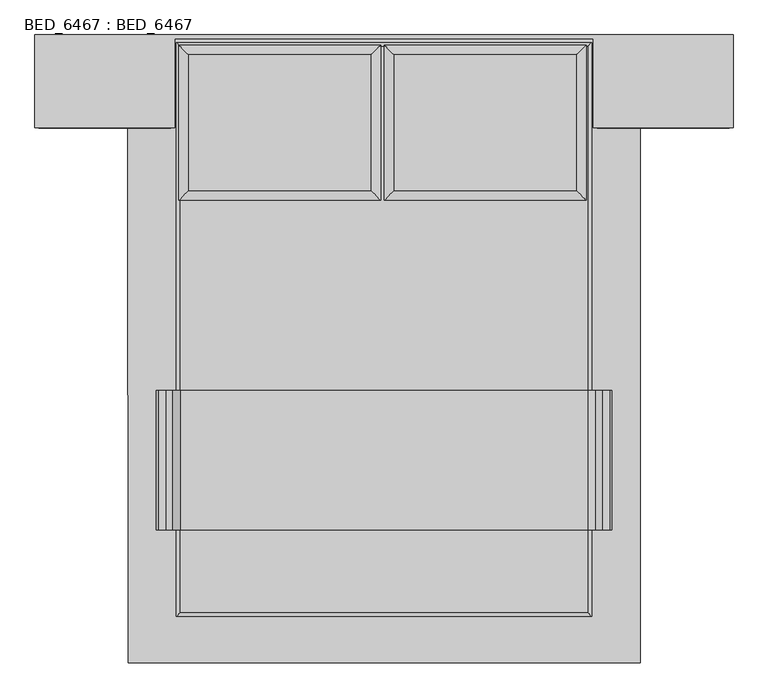
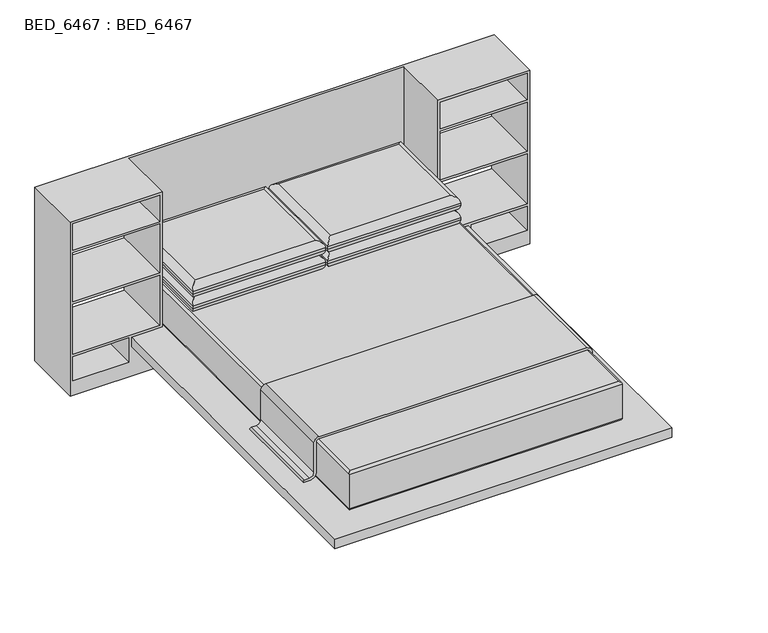
"""IFC4 building model written with IfcOpenShell, lengths in millimetres: proxy geometry, BED_6467 : BED_6467."""

from ifc_helpers import new_model, si_unit, point, frame, frame_2d, origin, place, context, project, spatial, polyline, circle_curve, ellipse_curve, trimmed, segment, composite_curve, outline, extrude, faceted_brep, source, transform, mapped, element, save
from ifc_brep_helpers import plane_surface, cylinder_surface, advanced_brep


def bed_6467_bed_6467_bd858abb(model_context):
    return source(origin(), model_context, "Body", "SolidModel", [
        advanced_brep(
        [(-695.3827629, -1070.2766054, 406.4), (638.1172371, -1070.2766054, 406.4), (638.1172371, 783.9233946, 406.4), (-695.3827629, 783.9233946, 406.4), (638.1172371, -1070.2766054, 203.2), (-695.3827629, -1070.2766054, 203.2), (-695.3827629, 783.9233946, 203.2), (638.1172371, 783.9233946, 203.2), (-708.0827629, -1082.9766054, 393.7), (-708.0827629, -1082.9766054, 215.9), (650.8172371, -1082.9766054, 215.9), (650.8172371, -1082.9766054, 393.7), (650.8172371, 796.6233946, 215.9), (650.8172371, 796.6233946, 393.7), (-708.0827629, 796.6233946, 215.9), (-708.0827629, 796.6233946, 393.7)],
        [
            (0, 1),
            (1, 2),
            (2, 3),
            (3, 0),
            (4, 5),
            (5, 6),
            (6, 7),
            (7, 4),
            (8, 9),
            (9, 10),
            (10, 11),
            (11, 8),
            (10, 12),
            (12, 13),
            (13, 11),
            (12, 14),
            (14, 15),
            (15, 13),
            (8, 15),
            (14, 9),
            (11, 1, ellipse_curve(frame((638.1172371, -1070.2766054, 393.7), z_axis=(-0.7071067811865475, -0.7071067811865475, 0.0), x_axis=(0.7071067811865476, -0.7071067811865474, 0.0)), 17.9605122, 12.7)),
            (0, 8, ellipse_curve(frame((-695.3827629, -1070.2766054, 393.7), z_axis=(0.7071067811865475, -0.7071067811865475, 0.0), x_axis=(0.7071067811865476, 0.7071067811865474, 0.0)), 17.9605122, 12.7)),
            (4, 10, ellipse_curve(frame((638.1172371, -1070.2766054, 215.9), z_axis=(-0.7071067811865475, -0.7071067811865475, 0.0), x_axis=(0.7071067811865476, -0.7071067811865474, 0.0)), 17.9605122, 12.7)),
            (9, 5, ellipse_curve(frame((-695.3827629, -1070.2766054, 215.9), z_axis=(0.7071067811865475, -0.7071067811865475, 0.0), x_axis=(0.7071067811865476, 0.7071067811865474, 0.0)), 17.9605122, 12.7)),
            (13, 2, ellipse_curve(frame((638.1172371, 783.9233946, 393.7), z_axis=(0.7071067811865475, -0.7071067811865475, 0.0), x_axis=(0.7071067811865474, 0.7071067811865476, 0.0)), 17.9605122, 12.7)),
            (7, 12, ellipse_curve(frame((638.1172371, 783.9233946, 215.9), z_axis=(0.7071067811865475, -0.7071067811865475, 0.0), x_axis=(0.7071067811865474, 0.7071067811865476, 0.0)), 17.9605122, 12.7)),
            (15, 3, ellipse_curve(frame((-695.3827629, 783.9233946, 393.7), z_axis=(0.7071067811865475, 0.7071067811865475, 0.0), x_axis=(-0.7071067811865476, 0.7071067811865474, 0.0)), 17.9605122, 12.7)),
            (6, 14, ellipse_curve(frame((-695.3827629, 783.9233946, 215.9), z_axis=(0.7071067811865475, 0.7071067811865475, 0.0), x_axis=(-0.7071067811865476, 0.7071067811865474, 0.0)), 17.9605122, 12.7)),
        ],
        [
            plane_surface(frame((-866.8327629, -1082.9766054, 406.4), z_axis=(0.0, 0.0, 1.0), x_axis=(1.0, 0.0, 0.0))),
            plane_surface(frame((-866.8327629, -1082.9766054, 203.2), z_axis=(0.0, 0.0, -1.0), x_axis=(-1.0, 0.0, 0.0))),
            plane_surface(frame((-708.0827629, -1082.9766054, 406.4), z_axis=(0.0, -1.0, 0.0), x_axis=(0.0, 0.0, -1.0))),
            plane_surface(frame((650.8172371, -1082.9766054, 406.4), z_axis=(1.0, 0.0, 0.0), x_axis=(0.0, 0.0, -1.0))),
            plane_surface(frame((650.8172371, 796.6233946, 406.4), z_axis=(0.0, 1.0, 0.0), x_axis=(0.0, 0.0, -1.0))),
            plane_surface(frame((-708.0827629, 796.6233946, 406.4), z_axis=(-1.0, 0.0, 0.0), x_axis=(0.0, 0.0, -1.0))),
            cylinder_surface(frame((-708.0827629, -1070.2766054, 393.7), z_axis=(1.0, 0.0, 0.0), x_axis=(0.0, 1.0, 0.0)), 12.7),
            cylinder_surface(frame((-708.0827629, -1070.2766054, 215.9), z_axis=(1.0, 0.0, 0.0), x_axis=(0.0, 1.0, 0.0)), 12.7),
            cylinder_surface(frame((638.1172371, -1082.9766054, 393.7), z_axis=(0.0, 1.0, 0.0), x_axis=(-1.0, 0.0, 0.0)), 12.7),
            cylinder_surface(frame((638.1172371, -1082.9766054, 215.9), z_axis=(0.0, 1.0, 0.0), x_axis=(-1.0, 0.0, 0.0)), 12.7),
            cylinder_surface(frame((650.8172371, 783.9233946, 393.7), z_axis=(-1.0, 0.0, 0.0), x_axis=(0.0, -1.0, 0.0)), 12.7),
            cylinder_surface(frame((650.8172371, 783.9233946, 215.9), z_axis=(-1.0, 0.0, 0.0), x_axis=(0.0, -1.0, 0.0)), 12.7),
            cylinder_surface(frame((-695.3827629, 796.6233946, 393.7), z_axis=(0.0, -1.0, 0.0), x_axis=(1.0, 0.0, 0.0)), 12.7),
            cylinder_surface(frame((-695.3827629, 796.6233946, 215.9), z_axis=(0.0, -1.0, 0.0), x_axis=(1.0, 0.0, 0.0)), 12.7),
        ],
        [
            (0, [[1, 2, 3, 4]]),
            (1, [[5, 6, 7, 8]]),
            (2, [[9, 10, 11, 12]]),
            (3, [[-11, 13, 14, 15]]),
            (4, [[-14, 16, 17, 18]]),
            (5, [[-9, 19, -17, 20]]),
            (6, [[21, -1, 22, -12]]),
            (7, [[23, -10, 24, -5]]),
            (8, [[-21, -15, 25, -2]]),
            (9, [[-23, -8, 26, -13]]),
            (10, [[-25, -18, 27, -3]]),
            (11, [[-26, -7, 28, -16]]),
            (12, [[-22, -4, -27, -19]]),
            (13, [[-24, -20, -28, -6]]),
        ],
    ),
        faceted_brep([(-714.4327629, 517.2233946, 914.4), (-714.4327629, 809.3233946, 914.4), (657.1672371, 809.3233946, 914.4), (657.1672371, 517.2233946, 914.4), (1114.3672371, 517.2233946, 914.4), (1114.3672371, 822.0233946, 914.4), (-1171.6327629, 822.0233946, 914.4), (-1171.6327629, 517.2233946, 914.4), (-714.4327629, 517.2233946, 0.0), (-1171.6327629, 517.2233946, 0.0), (-1171.6327629, 822.0233946, 0.0), (1114.3672371, 822.0233946, 0.0), (1114.3672371, 517.2233946, 0.0), (657.1672371, 517.2233946, 0.0), (657.1672371, 809.3233946, 0.0), (-714.4327629, 809.3233946, 0.0), (-714.4327629, 517.2233946, 203.2), (-714.4327629, 809.3233946, 203.2), (-714.4327629, 809.3233946, 152.4), (-714.4327629, 517.2233946, 152.4), (657.1672371, 809.3233946, 203.2), (657.1672371, 809.3233946, 152.4), (657.1672371, 517.2233946, 203.2), (657.1672371, 517.2233946, 152.4), (809.5672371, 517.2233946, 203.2), (809.5672371, 517.2233946, 152.4), (822.2672371, 517.2233946, 203.2), (1101.6672371, 517.2233946, 203.2), (1101.6672371, 517.2233946, 76.2), (822.2672371, 517.2233946, 76.2), (669.8672371, 517.2233946, 762.0), (669.8672371, 517.2233946, 901.7), (1101.6672371, 517.2233946, 901.7), (1101.6672371, 517.2233946, 762.0), (1101.6672371, 517.2233946, 479.0089549), (1101.6672371, 517.2233946, 215.9), (669.8672371, 517.2233946, 215.9), (669.8672371, 517.2233946, 479.0089549), (1101.6672371, 517.2233946, 749.3), (1101.6672371, 517.2233946, 491.7089549), (669.8672371, 517.2233946, 491.7089549), (669.8672371, 517.2233946, 749.3), (-1158.9327629, 822.0233946, 203.2), (-1158.9327629, 822.0233946, 76.2), (-879.5327629, 822.0233946, 76.2), (-879.5327629, 822.0233946, 203.2), (-1158.9327629, 822.0233946, 215.9), (-727.1327629, 822.0233946, 215.9), (-727.1327629, 822.0233946, 479.0089549), (-1158.9327629, 822.0233946, 479.0089549), (-727.1327629, 822.0233946, 901.7), (-1158.9327629, 822.0233946, 901.7), (-1158.9327629, 822.0233946, 762.0), (-727.1327629, 822.0233946, 762.0), (-1158.9327629, 822.0233946, 491.7089549), (-727.1327629, 822.0233946, 491.7089549), (-727.1327629, 822.0233946, 749.3), (-1158.9327629, 822.0233946, 749.3), (1101.6672371, 822.0233946, 203.2), (822.2672371, 822.0233946, 203.2), (822.2672371, 822.0233946, 76.2), (1101.6672371, 822.0233946, 76.2), (669.8672371, 822.0233946, 901.7), (669.8672371, 822.0233946, 762.0), (1101.6672371, 822.0233946, 762.0), (1101.6672371, 822.0233946, 901.7), (1101.6672371, 822.0233946, 215.9), (1101.6672371, 822.0233946, 479.0089549), (669.8672371, 822.0233946, 479.0089549), (669.8672371, 822.0233946, 215.9), (1101.6672371, 822.0233946, 491.7089549), (1101.6672371, 822.0233946, 749.3), (669.8672371, 822.0233946, 749.3), (669.8672371, 822.0233946, 491.7089549), (-866.8327629, 517.2233946, 152.4), (-866.8327629, 517.2233946, 203.2), (-1158.9327629, 517.2233946, 76.2), (-1158.9327629, 517.2233946, 203.2), (-879.5327629, 517.2233946, 203.2), (-879.5327629, 517.2233946, 76.2), (-727.1327629, 517.2233946, 215.9), (-1158.9327629, 517.2233946, 215.9), (-1158.9327629, 517.2233946, 479.0089549), (-727.1327629, 517.2233946, 479.0089549), (-1158.9327629, 517.2233946, 901.7), (-727.1327629, 517.2233946, 901.7), (-727.1327629, 517.2233946, 762.0), (-1158.9327629, 517.2233946, 762.0), (-727.1327629, 517.2233946, 491.7089549), (-1158.9327629, 517.2233946, 491.7089549), (-1158.9327629, 517.2233946, 749.3), (-727.1327629, 517.2233946, 749.3), (-866.8327629, -1235.3766054, 203.2), (809.5672371, -1235.3766054, 203.2), (809.5672371, -1235.3766054, 152.4), (-866.8327629, -1235.3766054, 152.4), (-562.0327629, 796.6233946, 152.4), (-562.0327629, -1006.7766054, 152.4), (504.7672371, -1006.7766054, 152.4), (504.7672371, 796.6233946, 152.4), (-562.0327629, 796.6233946, 0.0), (504.7672371, 796.6233946, 0.0), (504.7672371, -1006.7766054, 0.0), (-562.0327629, -1006.7766054, 0.0)], [[[0, 1, 2, 3, 4, 5, 6, 7]], [[8, 9, 10, 11, 12, 13, 14, 15]], [[1, 0, 16, 17]], [[8, 15, 18, 19]], [[2, 1, 17, 20]], [[15, 14, 21, 18]], [[3, 2, 20, 22]], [[14, 13, 23, 21]], [[4, 3, 22, 24, 25, 23, 13, 12], [26, 27, 28, 29], [30, 31, 32, 33], [34, 35, 36, 37], [38, 39, 40, 41]], [[5, 4, 12, 11]], [[6, 5, 11, 10], [42, 43, 44, 45], [46, 47, 48, 49], [50, 51, 52, 53], [54, 55, 56, 57], [58, 59, 60, 61], [62, 63, 64, 65], [66, 67, 68, 69], [70, 71, 72, 73]], [[7, 6, 10, 9]], [[0, 7, 9, 8, 19, 74, 75, 16], [76, 77, 78, 79], [80, 81, 82, 83], [84, 85, 86, 87], [88, 89, 90, 91]], [[75, 92, 93, 24, 22, 20, 17, 16]], [[25, 94, 95, 74, 19, 18, 21, 23], [96, 97, 98, 99]], [[92, 75, 74, 95]], [[93, 92, 95, 94]], [[24, 93, 94, 25]], [[100, 101, 102, 103]], [[100, 103, 97, 96]], [[103, 102, 98, 97]], [[102, 101, 99, 98]], [[101, 100, 96, 99]], [[76, 43, 42, 77]], [[43, 76, 79, 44]], [[44, 79, 78, 45]], [[77, 42, 45, 78]], [[84, 51, 50, 85]], [[51, 84, 87, 52]], [[52, 87, 86, 53]], [[85, 50, 53, 86]], [[80, 47, 46, 81]], [[47, 80, 83, 48]], [[48, 83, 82, 49]], [[81, 46, 49, 82]], [[88, 55, 54, 89]], [[55, 88, 91, 56]], [[56, 91, 90, 57]], [[89, 54, 57, 90]], [[26, 59, 58, 27]], [[59, 26, 29, 60]], [[60, 29, 28, 61]], [[27, 58, 61, 28]], [[30, 63, 62, 31]], [[63, 30, 33, 64]], [[64, 33, 32, 65]], [[31, 62, 65, 32]], [[34, 67, 66, 35]], [[67, 34, 37, 68]], [[68, 37, 36, 69]], [[35, 66, 69, 36]], [[38, 71, 70, 39]], [[71, 38, 41, 72]], [[72, 41, 40, 73]], [[39, 70, 73, 40]]]),
        advanced_brep(
        [(-668.444163, 311.8406819, 482.6), (-71.544163, 311.8406819, 482.6), (-71.544163, 756.3406819, 482.6), (-668.444163, 756.3406819, 482.6), (-71.544163, 311.8406819, 406.4), (-668.444163, 311.8406819, 406.4), (-668.444163, 756.3406819, 406.4), (-71.544163, 756.3406819, 406.4), (-39.794163, 788.0906819, 450.85), (-39.794163, 788.0906819, 438.15), (-700.194163, 788.0906819, 438.15), (-700.194163, 788.0906819, 450.85), (-700.194163, 280.0906819, 438.15), (-700.194163, 280.0906819, 450.85), (-39.794163, 280.0906819, 438.15), (-39.794163, 280.0906819, 450.85)],
        [
            (0, 1),
            (1, 2),
            (2, 3),
            (3, 0),
            (4, 5),
            (5, 6),
            (6, 7),
            (7, 4),
            (8, 9),
            (9, 10),
            (10, 11),
            (11, 8),
            (10, 12),
            (12, 13),
            (13, 11),
            (12, 14),
            (14, 15),
            (15, 13),
            (8, 15),
            (14, 9),
            (15, 1, ellipse_curve(frame((-71.544163, 311.8406819, 450.85), z_axis=(-0.7071067811865475, -0.7071067811865475, 0.0), x_axis=(0.7071067811865476, -0.7071067811865474, 0.0)), 44.9012806, 31.75)),
            (0, 13, ellipse_curve(frame((-668.444163, 311.8406819, 450.85), z_axis=(0.7071067811865475, -0.7071067811865475, 0.0), x_axis=(0.7071067811865476, 0.7071067811865474, 0.0)), 44.9012806, 31.75)),
            (4, 14, ellipse_curve(frame((-71.544163, 311.8406819, 438.15), z_axis=(-0.7071067811865475, -0.7071067811865475, 0.0), x_axis=(0.7071067811865476, -0.7071067811865474, 0.0)), 44.9012806, 31.75)),
            (12, 5, ellipse_curve(frame((-668.444163, 311.8406819, 438.15), z_axis=(0.7071067811865475, -0.7071067811865475, 0.0), x_axis=(0.7071067811865476, 0.7071067811865474, 0.0)), 44.9012806, 31.75)),
            (8, 2, ellipse_curve(frame((-71.544163, 756.3406819, 450.85), z_axis=(0.7071067811865475, -0.7071067811865475, 0.0), x_axis=(0.7071067811865474, 0.7071067811865476, 0.0)), 44.9012806, 31.75)),
            (7, 9, ellipse_curve(frame((-71.544163, 756.3406819, 438.15), z_axis=(0.7071067811865475, -0.7071067811865475, 0.0), x_axis=(0.7071067811865474, 0.7071067811865476, 0.0)), 44.9012806, 31.75)),
            (11, 3, ellipse_curve(frame((-668.444163, 756.3406819, 450.85), z_axis=(0.7071067811865475, 0.7071067811865475, 0.0), x_axis=(-0.7071067811865476, 0.7071067811865474, 0.0)), 44.9012806, 31.75)),
            (6, 10, ellipse_curve(frame((-668.444163, 756.3406819, 438.15), z_axis=(0.7071067811865475, 0.7071067811865475, 0.0), x_axis=(-0.7071067811865476, 0.7071067811865474, 0.0)), 44.9012806, 31.75)),
        ],
        [
            plane_surface(frame((-700.194163, 788.0906819, 482.6), z_axis=(0.0, 0.0, 1.0), x_axis=(-1.0, 0.0, 0.0))),
            plane_surface(frame((-700.194163, 788.0906819, 406.4), z_axis=(0.0, 0.0, -1.0), x_axis=(1.0, 0.0, 0.0))),
            plane_surface(frame((-39.794163, 788.0906819, 482.6), z_axis=(0.0, 1.0, 0.0), x_axis=(0.0, 0.0, -1.0))),
            plane_surface(frame((-700.194163, 788.0906819, 482.6), z_axis=(-1.0, 0.0, 0.0), x_axis=(0.0, 0.0, -1.0))),
            plane_surface(frame((-700.194163, 280.0906819, 482.6), z_axis=(0.0, -1.0, 0.0), x_axis=(0.0, 0.0, -1.0))),
            plane_surface(frame((-39.794163, 280.0906819, 482.6), z_axis=(1.0, 0.0, 0.0), x_axis=(0.0, 0.0, -1.0))),
            cylinder_surface(frame((-700.194163, 311.8406819, 450.85), z_axis=(1.0, 0.0, 0.0), x_axis=(0.0, 1.0, 0.0)), 31.75),
            cylinder_surface(frame((-700.194163, 311.8406819, 438.15), z_axis=(1.0, 0.0, 0.0), x_axis=(0.0, 1.0, 0.0)), 31.75),
            cylinder_surface(frame((-71.544163, 280.0906819, 450.85), z_axis=(0.0, 1.0, 0.0), x_axis=(-1.0, 0.0, 0.0)), 31.75),
            cylinder_surface(frame((-71.544163, 280.0906819, 438.15), z_axis=(0.0, 1.0, 0.0), x_axis=(-1.0, 0.0, 0.0)), 31.75),
            cylinder_surface(frame((-39.794163, 756.3406819, 450.85), z_axis=(-1.0, 0.0, 0.0), x_axis=(0.0, -1.0, 0.0)), 31.75),
            cylinder_surface(frame((-39.794163, 756.3406819, 438.15), z_axis=(-1.0, 0.0, 0.0), x_axis=(0.0, -1.0, 0.0)), 31.75),
            cylinder_surface(frame((-668.444163, 788.0906819, 450.85), z_axis=(0.0, -1.0, 0.0), x_axis=(1.0, 0.0, 0.0)), 31.75),
            cylinder_surface(frame((-668.444163, 788.0906819, 438.15), z_axis=(0.0, -1.0, 0.0), x_axis=(1.0, 0.0, 0.0)), 31.75),
        ],
        [
            (0, [[1, 2, 3, 4]]),
            (1, [[5, 6, 7, 8]]),
            (2, [[9, 10, 11, 12]]),
            (3, [[-11, 13, 14, 15]]),
            (4, [[-14, 16, 17, 18]]),
            (5, [[-9, 19, -17, 20]]),
            (6, [[21, -1, 22, -18]]),
            (7, [[23, -16, 24, -5]]),
            (8, [[-21, -19, 25, -2]]),
            (9, [[-23, -8, 26, -20]]),
            (10, [[-25, -12, 27, -3]]),
            (11, [[-26, -7, 28, -10]]),
            (12, [[-22, -4, -27, -15]]),
            (13, [[-24, -13, -28, -6]]),
        ],
    ),
        advanced_brep(
        [(4.655837, 311.8406819, 482.6), (601.555837, 311.8406819, 482.6), (601.555837, 756.3406819, 482.6), (4.655837, 756.3406819, 482.6), (601.555837, 311.8406819, 406.4), (4.655837, 311.8406819, 406.4), (4.655837, 756.3406819, 406.4), (601.555837, 756.3406819, 406.4), (633.305837, 788.0906819, 450.85), (633.305837, 788.0906819, 438.15), (-27.094163, 788.0906819, 438.15), (-27.094163, 788.0906819, 450.85), (-27.094163, 280.0906819, 438.15), (-27.094163, 280.0906819, 450.85), (633.305837, 280.0906819, 438.15), (633.305837, 280.0906819, 450.85)],
        [
            (0, 1),
            (1, 2),
            (2, 3),
            (3, 0),
            (4, 5),
            (5, 6),
            (6, 7),
            (7, 4),
            (8, 9),
            (9, 10),
            (10, 11),
            (11, 8),
            (10, 12),
            (12, 13),
            (13, 11),
            (12, 14),
            (14, 15),
            (15, 13),
            (8, 15),
            (14, 9),
            (15, 1, ellipse_curve(frame((601.555837, 311.8406819, 450.85), z_axis=(-0.7071067811865475, -0.7071067811865475, 0.0), x_axis=(0.7071067811865476, -0.7071067811865474, 0.0)), 44.9012806, 31.75)),
            (0, 13, ellipse_curve(frame((4.655837, 311.8406819, 450.85), z_axis=(0.7071067811865475, -0.7071067811865475, 0.0), x_axis=(0.7071067811865476, 0.7071067811865474, 0.0)), 44.9012806, 31.75)),
            (4, 14, ellipse_curve(frame((601.555837, 311.8406819, 438.15), z_axis=(-0.7071067811865475, -0.7071067811865475, 0.0), x_axis=(0.7071067811865476, -0.7071067811865474, 0.0)), 44.9012806, 31.75)),
            (12, 5, ellipse_curve(frame((4.655837, 311.8406819, 438.15), z_axis=(0.7071067811865475, -0.7071067811865475, 0.0), x_axis=(0.7071067811865476, 0.7071067811865474, 0.0)), 44.9012806, 31.75)),
            (8, 2, ellipse_curve(frame((601.555837, 756.3406819, 450.85), z_axis=(0.7071067811865475, -0.7071067811865475, 0.0), x_axis=(0.7071067811865474, 0.7071067811865476, 0.0)), 44.9012806, 31.75)),
            (7, 9, ellipse_curve(frame((601.555837, 756.3406819, 438.15), z_axis=(0.7071067811865475, -0.7071067811865475, 0.0), x_axis=(0.7071067811865474, 0.7071067811865476, 0.0)), 44.9012806, 31.75)),
            (11, 3, ellipse_curve(frame((4.655837, 756.3406819, 450.85), z_axis=(0.7071067811865475, 0.7071067811865475, 0.0), x_axis=(-0.7071067811865476, 0.7071067811865474, 0.0)), 44.9012806, 31.75)),
            (6, 10, ellipse_curve(frame((4.655837, 756.3406819, 438.15), z_axis=(0.7071067811865475, 0.7071067811865475, 0.0), x_axis=(-0.7071067811865476, 0.7071067811865474, 0.0)), 44.9012806, 31.75)),
        ],
        [
            plane_surface(frame((-27.094163, 788.0906819, 482.6), z_axis=(0.0, 0.0, 1.0), x_axis=(-1.0, 0.0, 0.0))),
            plane_surface(frame((-27.094163, 788.0906819, 406.4), z_axis=(0.0, 0.0, -1.0), x_axis=(1.0, 0.0, 0.0))),
            plane_surface(frame((633.305837, 788.0906819, 482.6), z_axis=(0.0, 1.0, 0.0), x_axis=(0.0, 0.0, -1.0))),
            plane_surface(frame((-27.094163, 788.0906819, 482.6), z_axis=(-1.0, 0.0, 0.0), x_axis=(0.0, 0.0, -1.0))),
            plane_surface(frame((-27.094163, 280.0906819, 482.6), z_axis=(0.0, -1.0, 0.0), x_axis=(0.0, 0.0, -1.0))),
            plane_surface(frame((633.305837, 280.0906819, 482.6), z_axis=(1.0, 0.0, 0.0), x_axis=(0.0, 0.0, -1.0))),
            cylinder_surface(frame((-27.094163, 311.8406819, 450.85), z_axis=(1.0, 0.0, 0.0), x_axis=(0.0, 1.0, 0.0)), 31.75),
            cylinder_surface(frame((-27.094163, 311.8406819, 438.15), z_axis=(1.0, 0.0, 0.0), x_axis=(0.0, 1.0, 0.0)), 31.75),
            cylinder_surface(frame((601.555837, 280.0906819, 450.85), z_axis=(0.0, 1.0, 0.0), x_axis=(-1.0, 0.0, 0.0)), 31.75),
            cylinder_surface(frame((601.555837, 280.0906819, 438.15), z_axis=(0.0, 1.0, 0.0), x_axis=(-1.0, 0.0, 0.0)), 31.75),
            cylinder_surface(frame((633.305837, 756.3406819, 450.85), z_axis=(-1.0, 0.0, 0.0), x_axis=(0.0, -1.0, 0.0)), 31.75),
            cylinder_surface(frame((633.305837, 756.3406819, 438.15), z_axis=(-1.0, 0.0, 0.0), x_axis=(0.0, -1.0, 0.0)), 31.75),
            cylinder_surface(frame((4.655837, 788.0906819, 450.85), z_axis=(0.0, -1.0, 0.0), x_axis=(1.0, 0.0, 0.0)), 31.75),
            cylinder_surface(frame((4.655837, 788.0906819, 438.15), z_axis=(0.0, -1.0, 0.0), x_axis=(1.0, 0.0, 0.0)), 31.75),
        ],
        [
            (0, [[1, 2, 3, 4]]),
            (1, [[5, 6, 7, 8]]),
            (2, [[9, 10, 11, 12]]),
            (3, [[-11, 13, 14, 15]]),
            (4, [[-14, 16, 17, 18]]),
            (5, [[-9, 19, -17, 20]]),
            (6, [[21, -1, 22, -18]]),
            (7, [[23, -16, 24, -5]]),
            (8, [[-21, -19, 25, -2]]),
            (9, [[-23, -8, 26, -20]]),
            (10, [[-25, -12, 27, -3]]),
            (11, [[-26, -7, 28, -10]]),
            (12, [[-22, -4, -27, -15]]),
            (13, [[-24, -13, -28, -6]]),
        ],
    ),
        advanced_brep(
        [(-668.444163, 311.8406819, 558.8), (-71.544163, 311.8406819, 558.8), (-71.544163, 756.3406819, 558.8), (-668.444163, 756.3406819, 558.8), (-71.544163, 311.8406819, 482.6), (-668.444163, 311.8406819, 482.6), (-668.444163, 756.3406819, 482.6), (-71.544163, 756.3406819, 482.6), (-39.794163, 788.0906819, 527.05), (-39.794163, 788.0906819, 514.35), (-700.194163, 788.0906819, 514.35), (-700.194163, 788.0906819, 527.05), (-700.194163, 280.0906819, 514.35), (-700.194163, 280.0906819, 527.05), (-39.794163, 280.0906819, 514.35), (-39.794163, 280.0906819, 527.05)],
        [
            (0, 1),
            (1, 2),
            (2, 3),
            (3, 0),
            (4, 5),
            (5, 6),
            (6, 7),
            (7, 4),
            (8, 9),
            (9, 10),
            (10, 11),
            (11, 8),
            (10, 12),
            (12, 13),
            (13, 11),
            (12, 14),
            (14, 15),
            (15, 13),
            (8, 15),
            (14, 9),
            (15, 1, ellipse_curve(frame((-71.544163, 311.8406819, 527.05), z_axis=(-0.7071067811865475, -0.7071067811865475, 0.0), x_axis=(0.7071067811865476, -0.7071067811865474, 0.0)), 44.9012806, 31.75)),
            (0, 13, ellipse_curve(frame((-668.444163, 311.8406819, 527.05), z_axis=(0.7071067811865475, -0.7071067811865475, 0.0), x_axis=(0.7071067811865476, 0.7071067811865474, 0.0)), 44.9012806, 31.75)),
            (4, 14, ellipse_curve(frame((-71.544163, 311.8406819, 514.35), z_axis=(-0.7071067811865475, -0.7071067811865475, 0.0), x_axis=(0.7071067811865476, -0.7071067811865474, 0.0)), 44.9012806, 31.75)),
            (12, 5, ellipse_curve(frame((-668.444163, 311.8406819, 514.35), z_axis=(0.7071067811865475, -0.7071067811865475, 0.0), x_axis=(0.7071067811865476, 0.7071067811865474, 0.0)), 44.9012806, 31.75)),
            (8, 2, ellipse_curve(frame((-71.544163, 756.3406819, 527.05), z_axis=(0.7071067811865475, -0.7071067811865475, 0.0), x_axis=(0.7071067811865474, 0.7071067811865476, 0.0)), 44.9012806, 31.75)),
            (7, 9, ellipse_curve(frame((-71.544163, 756.3406819, 514.35), z_axis=(0.7071067811865475, -0.7071067811865475, 0.0), x_axis=(0.7071067811865474, 0.7071067811865476, 0.0)), 44.9012806, 31.75)),
            (11, 3, ellipse_curve(frame((-668.444163, 756.3406819, 527.05), z_axis=(0.7071067811865475, 0.7071067811865475, 0.0), x_axis=(-0.7071067811865476, 0.7071067811865474, 0.0)), 44.9012806, 31.75)),
            (6, 10, ellipse_curve(frame((-668.444163, 756.3406819, 514.35), z_axis=(0.7071067811865475, 0.7071067811865475, 0.0), x_axis=(-0.7071067811865476, 0.7071067811865474, 0.0)), 44.9012806, 31.75)),
        ],
        [
            plane_surface(frame((-700.194163, 788.0906819, 558.8), z_axis=(0.0, 0.0, 1.0), x_axis=(-1.0, 0.0, 0.0))),
            plane_surface(frame((-700.194163, 788.0906819, 482.6), z_axis=(0.0, 0.0, -1.0), x_axis=(1.0, 0.0, 0.0))),
            plane_surface(frame((-39.794163, 788.0906819, 558.8), z_axis=(0.0, 1.0, 0.0), x_axis=(0.0, 0.0, -1.0))),
            plane_surface(frame((-700.194163, 788.0906819, 558.8), z_axis=(-1.0, 0.0, 0.0), x_axis=(0.0, 0.0, -1.0))),
            plane_surface(frame((-700.194163, 280.0906819, 558.8), z_axis=(0.0, -1.0, 0.0), x_axis=(0.0, 0.0, -1.0))),
            plane_surface(frame((-39.794163, 280.0906819, 558.8), z_axis=(1.0, 0.0, 0.0), x_axis=(0.0, 0.0, -1.0))),
            cylinder_surface(frame((-700.194163, 311.8406819, 527.05), z_axis=(1.0, 0.0, 0.0), x_axis=(0.0, 1.0, 0.0)), 31.75),
            cylinder_surface(frame((-700.194163, 311.8406819, 514.35), z_axis=(1.0, 0.0, 0.0), x_axis=(0.0, 1.0, 0.0)), 31.75),
            cylinder_surface(frame((-71.544163, 280.0906819, 527.05), z_axis=(0.0, 1.0, 0.0), x_axis=(-1.0, 0.0, 0.0)), 31.75),
            cylinder_surface(frame((-71.544163, 280.0906819, 514.35), z_axis=(0.0, 1.0, 0.0), x_axis=(-1.0, 0.0, 0.0)), 31.75),
            cylinder_surface(frame((-39.794163, 756.3406819, 527.05), z_axis=(-1.0, 0.0, 0.0), x_axis=(0.0, -1.0, 0.0)), 31.75),
            cylinder_surface(frame((-39.794163, 756.3406819, 514.35), z_axis=(-1.0, 0.0, 0.0), x_axis=(0.0, -1.0, 0.0)), 31.75),
            cylinder_surface(frame((-668.444163, 788.0906819, 527.05), z_axis=(0.0, -1.0, 0.0), x_axis=(1.0, 0.0, 0.0)), 31.75),
            cylinder_surface(frame((-668.444163, 788.0906819, 514.35), z_axis=(0.0, -1.0, 0.0), x_axis=(1.0, 0.0, 0.0)), 31.75),
        ],
        [
            (0, [[1, 2, 3, 4]]),
            (1, [[5, 6, 7, 8]]),
            (2, [[9, 10, 11, 12]]),
            (3, [[-11, 13, 14, 15]]),
            (4, [[-14, 16, 17, 18]]),
            (5, [[-9, 19, -17, 20]]),
            (6, [[21, -1, 22, -18]]),
            (7, [[23, -16, 24, -5]]),
            (8, [[-21, -19, 25, -2]]),
            (9, [[-23, -8, 26, -20]]),
            (10, [[-25, -12, 27, -3]]),
            (11, [[-26, -7, 28, -10]]),
            (12, [[-22, -4, -27, -15]]),
            (13, [[-24, -13, -28, -6]]),
        ],
    ),
        advanced_brep(
        [(4.655837, 311.8406819, 558.8), (601.555837, 311.8406819, 558.8), (601.555837, 756.3406819, 558.8), (4.655837, 756.3406819, 558.8), (601.555837, 311.8406819, 482.6), (4.655837, 311.8406819, 482.6), (4.655837, 756.3406819, 482.6), (601.555837, 756.3406819, 482.6), (633.305837, 788.0906819, 527.05), (633.305837, 788.0906819, 514.35), (-27.094163, 788.0906819, 514.35), (-27.094163, 788.0906819, 527.05), (-27.094163, 280.0906819, 514.35), (-27.094163, 280.0906819, 527.05), (633.305837, 280.0906819, 514.35), (633.305837, 280.0906819, 527.05)],
        [
            (0, 1),
            (1, 2),
            (2, 3),
            (3, 0),
            (4, 5),
            (5, 6),
            (6, 7),
            (7, 4),
            (8, 9),
            (9, 10),
            (10, 11),
            (11, 8),
            (10, 12),
            (12, 13),
            (13, 11),
            (12, 14),
            (14, 15),
            (15, 13),
            (8, 15),
            (14, 9),
            (15, 1, ellipse_curve(frame((601.555837, 311.8406819, 527.05), z_axis=(-0.7071067811865475, -0.7071067811865475, 0.0), x_axis=(0.7071067811865476, -0.7071067811865474, 0.0)), 44.9012806, 31.75)),
            (0, 13, ellipse_curve(frame((4.655837, 311.8406819, 527.05), z_axis=(0.7071067811865475, -0.7071067811865475, 0.0), x_axis=(0.7071067811865476, 0.7071067811865474, 0.0)), 44.9012806, 31.75)),
            (4, 14, ellipse_curve(frame((601.555837, 311.8406819, 514.35), z_axis=(-0.7071067811865475, -0.7071067811865475, 0.0), x_axis=(0.7071067811865476, -0.7071067811865474, 0.0)), 44.9012806, 31.75)),
            (12, 5, ellipse_curve(frame((4.655837, 311.8406819, 514.35), z_axis=(0.7071067811865475, -0.7071067811865475, 0.0), x_axis=(0.7071067811865476, 0.7071067811865474, 0.0)), 44.9012806, 31.75)),
            (8, 2, ellipse_curve(frame((601.555837, 756.3406819, 527.05), z_axis=(0.7071067811865475, -0.7071067811865475, 0.0), x_axis=(0.7071067811865474, 0.7071067811865476, 0.0)), 44.9012806, 31.75)),
            (7, 9, ellipse_curve(frame((601.555837, 756.3406819, 514.35), z_axis=(0.7071067811865475, -0.7071067811865475, 0.0), x_axis=(0.7071067811865474, 0.7071067811865476, 0.0)), 44.9012806, 31.75)),
            (11, 3, ellipse_curve(frame((4.655837, 756.3406819, 527.05), z_axis=(0.7071067811865475, 0.7071067811865475, 0.0), x_axis=(-0.7071067811865476, 0.7071067811865474, 0.0)), 44.9012806, 31.75)),
            (6, 10, ellipse_curve(frame((4.655837, 756.3406819, 514.35), z_axis=(0.7071067811865475, 0.7071067811865475, 0.0), x_axis=(-0.7071067811865476, 0.7071067811865474, 0.0)), 44.9012806, 31.75)),
        ],
        [
            plane_surface(frame((-27.094163, 788.0906819, 558.8), z_axis=(0.0, 0.0, 1.0), x_axis=(-1.0, 0.0, 0.0))),
            plane_surface(frame((-27.094163, 788.0906819, 482.6), z_axis=(0.0, 0.0, -1.0), x_axis=(1.0, 0.0, 0.0))),
            plane_surface(frame((633.305837, 788.0906819, 558.8), z_axis=(0.0, 1.0, 0.0), x_axis=(0.0, 0.0, -1.0))),
            plane_surface(frame((-27.094163, 788.0906819, 558.8), z_axis=(-1.0, 0.0, 0.0), x_axis=(0.0, 0.0, -1.0))),
            plane_surface(frame((-27.094163, 280.0906819, 558.8), z_axis=(0.0, -1.0, 0.0), x_axis=(0.0, 0.0, -1.0))),
            plane_surface(frame((633.305837, 280.0906819, 558.8), z_axis=(1.0, 0.0, 0.0), x_axis=(0.0, 0.0, -1.0))),
            cylinder_surface(frame((-27.094163, 311.8406819, 527.05), z_axis=(1.0, 0.0, 0.0), x_axis=(0.0, 1.0, 0.0)), 31.75),
            cylinder_surface(frame((-27.094163, 311.8406819, 514.35), z_axis=(1.0, 0.0, 0.0), x_axis=(0.0, 1.0, 0.0)), 31.75),
            cylinder_surface(frame((601.555837, 280.0906819, 527.05), z_axis=(0.0, 1.0, 0.0), x_axis=(-1.0, 0.0, 0.0)), 31.75),
            cylinder_surface(frame((601.555837, 280.0906819, 514.35), z_axis=(0.0, 1.0, 0.0), x_axis=(-1.0, 0.0, 0.0)), 31.75),
            cylinder_surface(frame((633.305837, 756.3406819, 527.05), z_axis=(-1.0, 0.0, 0.0), x_axis=(0.0, -1.0, 0.0)), 31.75),
            cylinder_surface(frame((633.305837, 756.3406819, 514.35), z_axis=(-1.0, 0.0, 0.0), x_axis=(0.0, -1.0, 0.0)), 31.75),
            cylinder_surface(frame((4.655837, 788.0906819, 527.05), z_axis=(0.0, -1.0, 0.0), x_axis=(1.0, 0.0, 0.0)), 31.75),
            cylinder_surface(frame((4.655837, 788.0906819, 514.35), z_axis=(0.0, -1.0, 0.0), x_axis=(1.0, 0.0, 0.0)), 31.75),
        ],
        [
            (0, [[1, 2, 3, 4]]),
            (1, [[5, 6, 7, 8]]),
            (2, [[9, 10, 11, 12]]),
            (3, [[-11, 13, 14, 15]]),
            (4, [[-14, 16, 17, 18]]),
            (5, [[-9, 19, -17, 20]]),
            (6, [[21, -1, 22, -18]]),
            (7, [[23, -16, 24, -5]]),
            (8, [[-21, -19, 25, -2]]),
            (9, [[-23, -8, 26, -20]]),
            (10, [[-25, -12, 27, -3]]),
            (11, [[-26, -7, 28, -10]]),
            (12, [[-22, -4, -27, -15]]),
            (13, [[-24, -13, -28, -6]]),
        ],
    ),
        extrude(outline(composite_curve([segment(trimmed(circle_curve(frame_2d((393.7, -695.3827629)), 12.7), [point((393.7, -708.0827629))], [point((406.4, -695.3827629))], True, "CARTESIAN"), True, "CONTINUOUS"), segment(polyline([(406.4, -695.3827629), (406.4, 638.1172371)]), True, "CONTINUOUS"), segment(trimmed(circle_curve(frame_2d((393.7, 638.1172371)), 12.7), [point((406.4, 638.1172371))], [point((393.7, 650.8172371))], True, "CARTESIAN"), True, "CONTINUOUS"), segment(polyline([(393.7, 650.8172371), (238.548362, 650.8172371)]), True, "CONTINUOUS"), segment(trimmed(circle_curve(frame_2d((238.548362, 686.1655991)), 35.348362), [point((238.548362, 650.8172371))], [point((203.2, 686.1655991))], False, "CARTESIAN"), True, "CONTINUOUS"), segment(polyline([(203.2, 686.1655991), (203.2, 710.6172368)]), True, "CONTINUOUS"), segment(trimmed(circle_curve(frame_2d((209.55, 710.6172368)), 6.35), [point((203.2, 710.6172368))], [point((215.9, 710.6172368))], False, "CARTESIAN"), True, "CONTINUOUS"), segment(polyline([(215.9, 710.6172368), (215.9, 686.1655991)]), True, "CONTINUOUS"), segment(trimmed(circle_curve(frame_2d((238.548362, 686.1655991)), 22.648362), [point((215.9, 686.1655991))], [point((238.548362, 663.5172371))], True, "CARTESIAN"), True, "CONTINUOUS"), segment(polyline([(238.548362, 663.5172371), (393.7, 663.5172371)]), True, "CONTINUOUS"), segment(trimmed(circle_curve(frame_2d((393.7, 638.1172371)), 25.4), [point((393.7, 663.5172371))], [point((419.1, 638.1172371))], False, "CARTESIAN"), True, "CONTINUOUS"), segment(polyline([(419.1, 638.1172371), (419.1, -695.3827629)]), True, "CONTINUOUS"), segment(trimmed(circle_curve(frame_2d((393.7, -695.3827629)), 25.4), [point((419.1, -695.3827629))], [point((393.7, -720.7827629))], False, "CARTESIAN"), True, "CONTINUOUS"), segment(polyline([(393.7, -720.7827629), (238.548362, -720.7827629)]), True, "CONTINUOUS"), segment(trimmed(circle_curve(frame_2d((238.548362, -743.4311248)), 22.648362), [point((238.548362, -720.7827629))], [point((215.9, -743.4311248))], True, "CARTESIAN"), True, "CONTINUOUS"), segment(polyline([(215.9, -743.4311248), (215.9, -767.8827625)]), True, "CONTINUOUS"), segment(trimmed(circle_curve(frame_2d((209.55, -767.8827625)), 6.35), [point((215.9, -767.8827625))], [point((203.2, -767.8827625))], False, "CARTESIAN"), True, "CONTINUOUS"), segment(polyline([(203.2, -767.8827625), (203.2, -743.4311248)]), True, "CONTINUOUS"), segment(trimmed(circle_curve(frame_2d((238.548362, -743.4311248)), 35.348362), [point((203.2, -743.4311248))], [point((238.548362, -708.0827629))], False, "CARTESIAN"), True, "CONTINUOUS"), segment(polyline([(238.548362, -708.0827629), (393.7, -708.0827629)]), True, "CONTINUOUS")], self_intersect=False)), frame((0.0, -800.4016054, 0.0), z_axis=(0.0, 1.0, 0.0), x_axis=(0.0, 0.0, 1.0)), (0.0, 0.0, 1.0), 457.2),
    ])


if __name__ == "__main__":
    model = new_model("IFC4")
    model_context = context("Model", 3, world=origin())
    ifc_project = project(units=[si_unit("LENGTHUNIT", "METRE", prefix="MILLI")], contexts=[model_context])
    site = spatial("IfcSite", under=ifc_project)
    building = spatial("IfcBuilding", under=site)
    placement = place(None, origin())
    bed_6467_bed_6467_shape = bed_6467_bed_6467_bd858abb(model_context)
    element("IfcBuildingElementProxy", 1, Name="BED_6467 : BED_6467", ObjectType="BED_6467 : BED_6467", at=placement, inside=building, context=model_context, shape_type="MappedRepresentation", body=[
        mapped(bed_6467_bed_6467_shape, transform((0.0, 0.0, 0.0), x_axis=(1.0, 0.0, 0.0), y_axis=(0.0, 1.0, 0.0), z_axis=(0.0, 0.0, 1.0))),
    ])
    save(model, "model.ifc")

# Revit data of these elements
# Type "BED_6467 : BED_6467"
#   Sheets [instance default] = Sheets
#   Pillow Set 2 [instance default] = Pillow 2
#   Pillow Set 1 [instance default] = Pillow 1
#   FRAME [instance default] = FRAME
#   Default Elevation = 0
# Element 1 (IfcBuildingElementProxy, "BED_6467 : BED_6467")
#   Materials on its faces: "FRAME", "Pillow 1", "Pillow 2", "Sheets"
# Materials
#   "Sheets": class "Fabric", colour RGB 255 255 255, transparency 0
#   "Pillow 2": class "Fabric", colour RGB 255 255 255, transparency 0
#   "Pillow 1": class "Fabric", colour RGB 0 64 128, transparency 0
#   "FRAME": class "Paint", colour RGB 58 58 58, transparency 0
